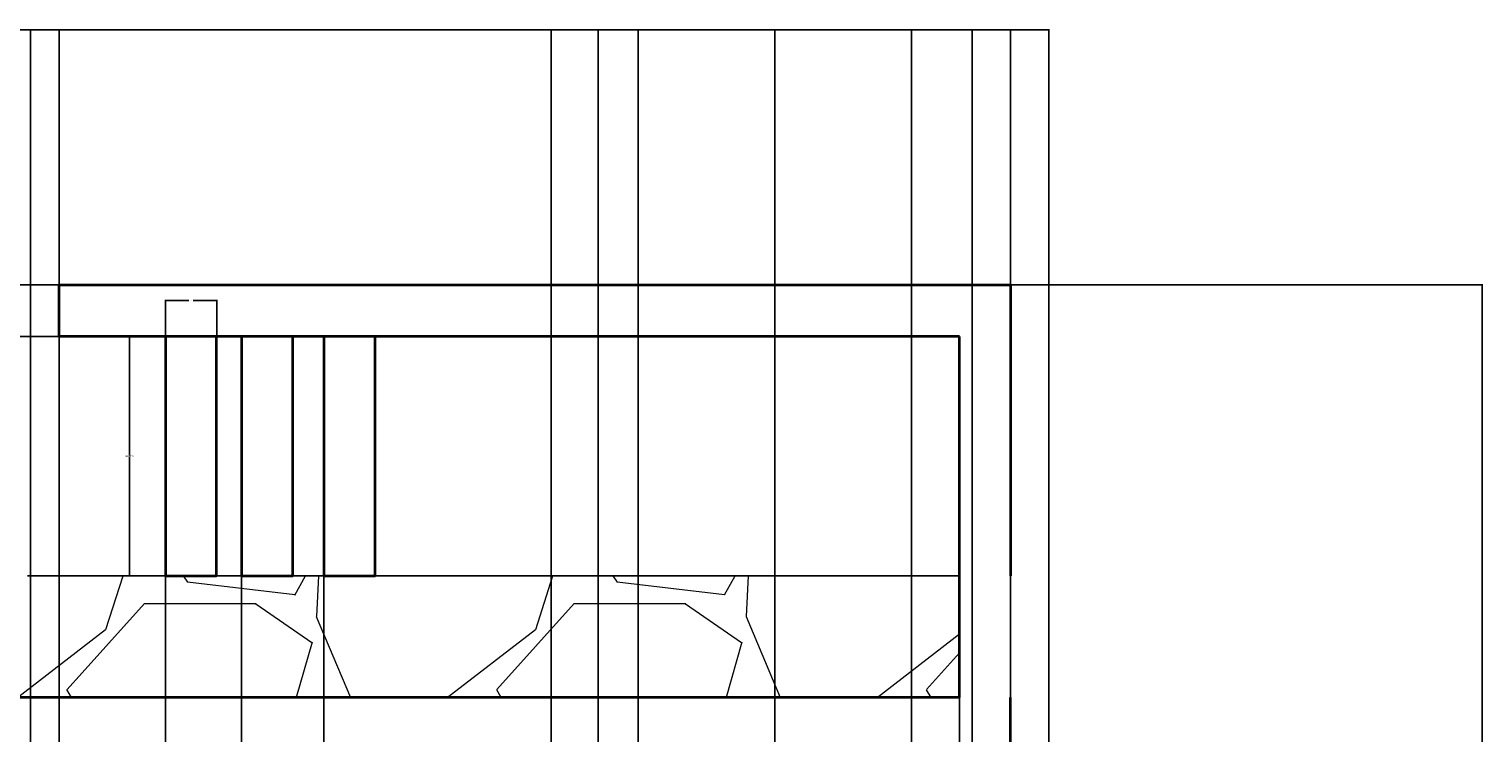
# Model space of a CAD drawing. Units: inches. Extents: x -8 to 554, y -200 to 499.
# Tile 12 of 12: x 216 to 554, y 335 to 499. Entities that reach past the tile are written whole.
import ezdxf

# ---------------------------------------------------------------- set-up
doc = ezdxf.new("R2010")
doc.units = ezdxf.units.IN
doc.header["$MEASUREMENT"] = 0
for name, color, linetype, lineweight in [('A-ANNO-DIMS', 2, 'Continuous', 18), ('A-FLOR', 7, 'Continuous', 35), ('A-ROOF', 7, 'Continuous', 35), ('A-WALL', 7, 'Continuous', 35), ('A-WALL-PATT', 252, 'Continuous', 13), ('A-WALL-PRPT', 7, 'Continuous', 25)]:
    doc.layers.add(name, color=color, linetype=linetype, lineweight=lineweight)
doc.styles.get("Standard").update_dxf_attribs({"font": 'arial.ttf'})
doc.dimstyles.get("Standard").update_dxf_attribs({"dimtxt": 0.18, "dimasz": 0.18, "dimexe": 0.18, "dimexo": 0.0625, "dimgap": 0.09, "dimtad": 0, "dimtih": 1, "dimtoh": 1, "dimdec": 4, "dimzin": 0, "dimdsep": 46, "dimtxsty": 'Standard', "dimcen": 0.09, "dimadec": 0, "dimazin": 0, "dimtfac": 1, "dimtdec": 4, "dimtofl": 0, "dimtmove": 0, "dimatfit": 3, "dimfxl": 1, "dimtolj": 1, "dimtzin": 0, "dimarcsym": 0})

# ---------------------------------------------------------------- blocks, each defined once
blk = doc.blocks.new('ROOF-UPRIGHT-ELEV')
blk.add_lwpolyline([(0, 0), (11.94, 0), (11.94, 55.69), (0, 55.69)], close=True)
blk = doc.blocks.new('*D22')
at = {"layer": 'A-ANNO-DIMS', "color": 0, "lineweight": -2, "transparency": 16777216}
for p, q in [((247.65, 427.48), (239.18, 427.48)), ((239.36, 427.3), (239.36, 399.82)), ((239.36, 371.97), (239.36, 399.45)), ((247.65, 371.79), (239.18, 371.79))]:
    blk.add_line(p, q, dxfattribs=at)
at = {"layer": 'A-ANNO-DIMS', "color": 0, "transparency": 16777216}
for points in [[(239.33, 427.3), (239.39, 427.3), (239.36, 427.48)], [(239.33, 371.97), (239.39, 371.97), (239.36, 371.79)]]:
    blk.add_solid(points, dxfattribs=at)
at = {"layer": 'Defpoints', "color": 0, "transparency": 16777216}
for p in [(239.36, 427.48), (247.72, 427.48), (247.72, 371.79)]:
    blk.add_point(p, dxfattribs=at)
at = {"layer": 'A-ANNO-DIMS', "color": 0, "transparency": 16777216, "insert": (239.36, 399.64), "char_height": 0.18, "attachment_point": 5}
blk.add_mtext('\\A1;UPRIGHT 56 TYP.', dxfattribs=at)
blk = doc.blocks.new('*D23')
at = {"layer": 'A-ANNO-DIMS', "color": 0, "lineweight": -2, "transparency": 16777216}
for p, q in [((247.72, 427.54), (247.72, 436.01)), ((247.9, 435.83), (253.17, 435.83)), ((259.48, 435.83), (254.21, 435.83)), ((259.66, 427.54), (259.66, 436.01))]:
    blk.add_line(p, q, dxfattribs=at)
at = {"layer": 'A-ANNO-DIMS', "color": 0, "transparency": 16777216}
for points in [[(247.9, 435.86), (247.9, 435.8), (247.72, 435.83)], [(259.48, 435.86), (259.48, 435.8), (259.66, 435.83)]]:
    blk.add_solid(points, dxfattribs=at)
at = {"layer": 'Defpoints', "color": 0, "transparency": 16777216}
for p in [(259.66, 435.83), (247.72, 427.48), (259.66, 427.48)]:
    blk.add_point(p, dxfattribs=at)
at = {"layer": 'A-ANNO-DIMS', "color": 0, "transparency": 16777216, "insert": (253.69, 435.83), "char_height": 0.18, "attachment_point": 5}
blk.add_mtext('\\A1;12 TYP.', dxfattribs=at)
blk = doc.blocks.new('*D30')
at = {"layer": 'A-ANNO-DIMS', "color": 0, "lineweight": -2, "transparency": 16777216}
for p, q in [((444.4, 439.48), (554.26, 439.48)), ((554.08, 439.3), (554.08, 163.66)), ((554.08, -112.34), (554.08, 163.3)), ((446.15, -112.52), (554.26, -112.52))]:
    blk.add_line(p, q, dxfattribs=at)
at = {"layer": 'A-ANNO-DIMS', "color": 0, "transparency": 16777216}
for points in [[(554.05, 439.3), (554.11, 439.3), (554.08, 439.48)], [(554.05, -112.34), (554.11, -112.34), (554.08, -112.52)]]:
    blk.add_solid(points, dxfattribs=at)
at = {"layer": 'Defpoints', "color": 0, "transparency": 16777216}
for p in [(444.34, 439.48), (446.09, -112.52), (554.08, -112.52)]:
    blk.add_point(p, dxfattribs=at)
at = {"layer": 'A-ANNO-DIMS', "color": 0, "transparency": 16777216, "insert": (554.08, 163.48), "char_height": 0.18, "attachment_point": 5}
blk.add_mtext('\\A1;552', dxfattribs=at)
blk = doc.blocks.new('*D39')
at = {"layer": 'A-ANNO-DIMS', "color": 0, "lineweight": -2, "transparency": 16777216}
for p, q in [((223.01, 439.54), (223.01, 498.99)), ((223.19, 498.81), (333.21, 498.81)), ((444.16, 498.81), (334.14, 498.81)), ((444.34, 439.54), (444.34, 498.99))]:
    blk.add_line(p, q, dxfattribs=at)
at = {"layer": 'A-ANNO-DIMS', "color": 0, "transparency": 16777216}
for points in [[(223.19, 498.84), (223.19, 498.78), (223.01, 498.81)], [(444.16, 498.84), (444.16, 498.78), (444.34, 498.81)]]:
    blk.add_solid(points, dxfattribs=at)
at = {"layer": 'Defpoints', "color": 0, "transparency": 16777216}
for p in [(444.34, 498.81), (223.01, 439.48), (444.34, 439.48)]:
    blk.add_point(p, dxfattribs=at)
at = {"layer": 'A-ANNO-DIMS', "color": 0, "transparency": 16777216, "insert": (333.68, 498.81), "char_height": 0.18, "attachment_point": 5}
blk.add_mtext('\\A1;221.33', dxfattribs=at)
blk = doc.blocks.new('*D40')
at = {"layer": 'A-ANNO-DIMS', "color": 0, "lineweight": -2, "transparency": 16777216}
for p, q in [((222.95, 439.48), (-7.69, 439.48)), ((-7.51, 439.3), (-7.51, 433.66)), ((-7.51, 427.66), (-7.51, 433.3)), ((222.95, 427.48), (-7.69, 427.48))]:
    blk.add_line(p, q, dxfattribs=at)
at = {"layer": 'A-ANNO-DIMS', "color": 0, "transparency": 16777216}
for points in [[(-7.54, 439.3), (-7.48, 439.3), (-7.51, 439.48)], [(-7.54, 427.66), (-7.48, 427.66), (-7.51, 427.48)]]:
    blk.add_solid(points, dxfattribs=at)
at = {"layer": 'Defpoints', "color": 0, "transparency": 16777216}
for p in [(223.01, 439.48), (-7.51, 427.48), (223.01, 427.48)]:
    blk.add_point(p, dxfattribs=at)
at = {"layer": 'A-ANNO-DIMS', "color": 0, "transparency": 16777216, "insert": (-7.51, 433.48), "char_height": 0.18, "attachment_point": 5}
blk.add_mtext('\\A1;12', dxfattribs=at)
blk = doc.blocks.new('*D43')
at = {"layer": 'A-ANNO-DIMS', "color": 0, "lineweight": -2, "transparency": 16777216}
for p, q in [((168.34, 319.54), (168.34, 498.99)), ((168.52, 498.81), (192.12, 498.81)), ((216.16, 498.81), (192.56, 498.81)), ((216.34, 319.54), (216.34, 498.99))]:
    blk.add_line(p, q, dxfattribs=at)
at = {"layer": 'A-ANNO-DIMS', "color": 0, "transparency": 16777216}
for points in [[(168.52, 498.84), (168.52, 498.78), (168.34, 498.81)], [(216.16, 498.84), (216.16, 498.78), (216.34, 498.81)]]:
    blk.add_solid(points, dxfattribs=at)
at = {"layer": 'Defpoints', "color": 0, "transparency": 16777216}
for p in [(216.34, 498.81), (168.34, 319.48), (216.34, 319.48)]:
    blk.add_point(p, dxfattribs=at)
at = {"layer": 'A-ANNO-DIMS', "color": 0, "transparency": 16777216, "insert": (192.34, 498.81), "char_height": 0.18, "attachment_point": 5}
blk.add_mtext('\\A1;48', dxfattribs=at)
blk = doc.blocks.new('*D45')
at = {"layer": 'A-ANNO-DIMS', "color": 0, "lineweight": -2, "transparency": 16777216}
for p, q in [((357.7, 319.85), (357.7, 498.99)), ((357.88, 498.81), (373.22, 498.81)), ((389.34, 498.81), (374, 498.81)), ((389.52, 319.54), (389.52, 498.99))]:
    blk.add_line(p, q, dxfattribs=at)
at = {"layer": 'A-ANNO-DIMS', "color": 0, "transparency": 16777216}
for points in [[(357.88, 498.84), (357.88, 498.78), (357.7, 498.81)], [(389.34, 498.84), (389.34, 498.78), (389.52, 498.81)]]:
    blk.add_solid(points, dxfattribs=at)
at = {"layer": 'Defpoints', "color": 0, "transparency": 16777216}
for p in [(389.52, 498.81), (357.7, 319.79), (389.52, 319.48)]:
    blk.add_point(p, dxfattribs=at)
at = {"layer": 'A-ANNO-DIMS', "color": 0, "transparency": 16777216, "insert": (373.61, 498.81), "char_height": 0.18, "attachment_point": 5}
blk.add_mtext('\\A1;31.82', dxfattribs=at)
blk = doc.blocks.new('*D55')
at = {"layer": 'A-ANNO-DIMS', "color": 0, "lineweight": -2, "transparency": 16777216}
for p, q in [((204.61, -30.61), (204.61, 498.99)), ((204.79, 498.81), (328.57, 498.81)), ((453.14, 498.81), (329.36, 498.81)), ((453.32, -30.61), (453.32, 498.99))]:
    blk.add_line(p, q, dxfattribs=at)
at = {"layer": 'A-ANNO-DIMS', "color": 0, "transparency": 16777216}
for points in [[(204.79, 498.84), (204.79, 498.78), (204.61, 498.81)], [(453.14, 498.84), (453.14, 498.78), (453.32, 498.81)]]:
    blk.add_solid(points, dxfattribs=at)
at = {"layer": 'Defpoints', "color": 0, "transparency": 16777216}
for p in [(453.32, 498.81), (204.61, -30.67), (453.32, -30.67)]:
    blk.add_point(p, dxfattribs=at)
at = {"layer": 'A-ANNO-DIMS', "color": 0, "transparency": 16777216, "insert": (328.96, 498.81), "char_height": 0.18, "attachment_point": 5}
blk.add_mtext('\\A1;248.7', dxfattribs=at)
blk = doc.blocks.new('*D62')
at = {"layer": 'A-ANNO-DIMS', "color": 0, "lineweight": -2, "transparency": 16777216}
for p, q in [((189.3, 7.54), (189.3, 498.99)), ((189.48, 498.81), (263.01, 498.81)), ((337.31, 498.81), (263.78, 498.81)), ((337.49, 7.54), (337.49, 498.99))]:
    blk.add_line(p, q, dxfattribs=at)
at = {"layer": 'A-ANNO-DIMS', "color": 0, "transparency": 16777216}
for points in [[(189.48, 498.84), (189.48, 498.78), (189.3, 498.81)], [(337.31, 498.84), (337.31, 498.78), (337.49, 498.81)]]:
    blk.add_solid(points, dxfattribs=at)
at = {"layer": 'Defpoints', "color": 0, "transparency": 16777216}
for p in [(337.49, 498.81), (189.3, 7.48), (337.49, 7.48)]:
    blk.add_point(p, dxfattribs=at)
at = {"layer": 'A-ANNO-DIMS', "color": 0, "transparency": 16777216, "insert": (263.4, 498.81), "char_height": 0.18, "attachment_point": 5}
blk.add_mtext('\\A1;148.2', dxfattribs=at)
blk = doc.blocks.new('*D63')
at = {"layer": 'A-ANNO-DIMS', "color": 0, "lineweight": -2, "transparency": 16777216}
for p, q in [((337.49, -52.76), (337.49, 498.99)), ((337.67, 498.81), (342.51, 498.81)), ((348.26, 498.81), (343.42, 498.81)), ((348.44, -52.76), (348.44, 498.99))]:
    blk.add_line(p, q, dxfattribs=at)
at = {"layer": 'A-ANNO-DIMS', "color": 0, "transparency": 16777216}
for points in [[(337.67, 498.84), (337.67, 498.78), (337.49, 498.81)], [(348.26, 498.84), (348.26, 498.78), (348.44, 498.81)]]:
    blk.add_solid(points, dxfattribs=at)
at = {"layer": 'Defpoints', "color": 0, "transparency": 16777216}
for p in [(348.44, 498.81), (337.49, -52.82), (348.44, -52.82)]:
    blk.add_point(p, dxfattribs=at)
at = {"layer": 'A-ANNO-DIMS', "color": 0, "transparency": 16777216, "insert": (342.97, 498.81), "char_height": 0.18, "attachment_point": 5}
blk.add_mtext('\\A1;10.946', dxfattribs=at)
blk = doc.blocks.new('*D64')
at = {"layer": 'A-ANNO-DIMS', "color": 0, "lineweight": -2, "transparency": 16777216}
for p, q in [((337.49, 7.54), (337.49, 498.99)), ((337.67, 498.81), (379.02, 498.81)), ((421.13, 498.81), (379.78, 498.81)), ((421.31, 7.54), (421.31, 498.99))]:
    blk.add_line(p, q, dxfattribs=at)
at = {"layer": 'A-ANNO-DIMS', "color": 0, "transparency": 16777216}
for points in [[(337.67, 498.84), (337.67, 498.78), (337.49, 498.81)], [(421.13, 498.84), (421.13, 498.78), (421.31, 498.81)]]:
    blk.add_solid(points, dxfattribs=at)
at = {"layer": 'Defpoints', "color": 0, "transparency": 16777216}
for p in [(421.31, 498.81), (337.49, 7.48), (421.31, 7.48)]:
    blk.add_point(p, dxfattribs=at)
at = {"layer": 'A-ANNO-DIMS', "color": 0, "transparency": 16777216, "insert": (379.4, 498.81), "char_height": 0.18, "attachment_point": 5}
blk.add_mtext('\\A1;83.81', dxfattribs=at)
blk = doc.blocks.new('*D65')
at = {"layer": 'A-ANNO-DIMS', "color": 0, "lineweight": -2, "transparency": 16777216}
for p, q in [((421.31, 7.54), (421.31, 498.99)), ((421.49, 498.81), (428, 498.81)), ((435.29, 498.81), (428.77, 498.81)), ((435.47, 7.54), (435.47, 498.99))]:
    blk.add_line(p, q, dxfattribs=at)
at = {"layer": 'A-ANNO-DIMS', "color": 0, "transparency": 16777216}
for points in [[(421.49, 498.84), (421.49, 498.78), (421.31, 498.81)], [(435.29, 498.84), (435.29, 498.78), (435.47, 498.81)]]:
    blk.add_solid(points, dxfattribs=at)
at = {"layer": 'Defpoints', "color": 0, "transparency": 16777216}
for p in [(435.47, 498.81), (421.31, 7.48), (435.47, 7.48)]:
    blk.add_point(p, dxfattribs=at)
at = {"layer": 'A-ANNO-DIMS', "color": 0, "transparency": 16777216, "insert": (428.39, 498.81), "char_height": 0.18, "attachment_point": 5}
blk.add_mtext('\\A1;14.16', dxfattribs=at)
blk = doc.blocks.new('*D67')
at = {"layer": 'A-ANNO-DIMS', "color": 0, "lineweight": -2, "transparency": 16777216}
for p, q in [((223.01, 427.42), (223.01, -199.97)), ((247.72, 427.42), (247.72, -199.97)), ((223.19, -199.79), (234.9, -199.79)), ((247.54, -199.79), (235.83, -199.79))]:
    blk.add_line(p, q, dxfattribs=at)
at = {"layer": 'A-ANNO-DIMS', "color": 0, "transparency": 16777216}
for points in [[(223.19, -199.76), (223.19, -199.82), (223.01, -199.79)], [(247.54, -199.76), (247.54, -199.82), (247.72, -199.79)]]:
    blk.add_solid(points, dxfattribs=at)
at = {"layer": 'Defpoints', "color": 0, "transparency": 16777216}
for p in [(223.01, 427.48), (247.72, 427.48), (247.72, -199.79)]:
    blk.add_point(p, dxfattribs=at)
at = {"layer": 'A-ANNO-DIMS', "color": 0, "transparency": 16777216, "insert": (235.36, -199.79), "char_height": 0.18, "attachment_point": 5}
blk.add_mtext('\\A1;24.705', dxfattribs=at)
blk = doc.blocks.new('*D68')
at = {"layer": 'A-ANNO-DIMS', "color": 0, "lineweight": -2, "transparency": 16777216}
for p, q in [((247.72, 371.73), (247.72, -199.97)), ((265.46, 371.73), (265.46, -199.97)), ((247.9, -199.79), (256.13, -199.79)), ((265.28, -199.79), (257.04, -199.79))]:
    blk.add_line(p, q, dxfattribs=at)
at = {"layer": 'A-ANNO-DIMS', "color": 0, "transparency": 16777216}
for points in [[(247.9, -199.76), (247.9, -199.82), (247.72, -199.79)], [(265.28, -199.76), (265.28, -199.82), (265.46, -199.79)]]:
    blk.add_solid(points, dxfattribs=at)
at = {"layer": 'Defpoints', "color": 0, "transparency": 16777216}
for p in [(247.72, 371.79), (265.46, 371.79), (265.46, -199.79)]:
    blk.add_point(p, dxfattribs=at)
at = {"layer": 'A-ANNO-DIMS', "color": 0, "transparency": 16777216, "insert": (256.59, -199.79), "char_height": 0.18, "attachment_point": 5}
blk.add_mtext('\\A1;17.744', dxfattribs=at)
blk = doc.blocks.new('*D69')
at = {"layer": 'A-ANNO-DIMS', "color": 0, "lineweight": -2, "transparency": 16777216}
for p, q in [((265.46, 371.73), (265.46, -199.97)), ((284.57, 371.73), (284.57, -199.97)), ((265.64, -199.79), (274.65, -199.79)), ((284.39, -199.79), (275.38, -199.79))]:
    blk.add_line(p, q, dxfattribs=at)
at = {"layer": 'A-ANNO-DIMS', "color": 0, "transparency": 16777216}
for points in [[(265.64, -199.76), (265.64, -199.82), (265.46, -199.79)], [(284.39, -199.76), (284.39, -199.82), (284.57, -199.79)]]:
    blk.add_solid(points, dxfattribs=at)
at = {"layer": 'Defpoints', "color": 0, "transparency": 16777216}
for p in [(265.46, 371.79), (284.57, 371.79), (284.57, -199.79)]:
    blk.add_point(p, dxfattribs=at)
at = {"layer": 'A-ANNO-DIMS', "color": 0, "transparency": 16777216, "insert": (275.01, -199.79), "char_height": 0.18, "attachment_point": 5}
blk.add_mtext('\\A1;19.11', dxfattribs=at)
blk = doc.blocks.new('*D71')
at = {"layer": 'A-ANNO-DIMS', "color": 0, "lineweight": -2, "transparency": 16777216}
for p, q in [((444.34, 439.42), (444.34, -199.97)), ((432.52, 427.42), (432.52, -199.97)), ((432.7, -199.79), (437.97, -199.79)), ((444.16, -199.79), (438.89, -199.79))]:
    blk.add_line(p, q, dxfattribs=at)
at = {"layer": 'A-ANNO-DIMS', "color": 0, "transparency": 16777216}
for points in [[(432.7, -199.76), (432.7, -199.82), (432.52, -199.79)], [(444.16, -199.76), (444.16, -199.82), (444.34, -199.79)]]:
    blk.add_solid(points, dxfattribs=at)
at = {"layer": 'Defpoints', "color": 0, "transparency": 16777216}
for p in [(444.34, 439.48), (432.52, 427.48), (444.34, -199.79)]:
    blk.add_point(p, dxfattribs=at)
at = {"layer": 'A-ANNO-DIMS', "color": 0, "transparency": 16777216, "insert": (438.43, -199.79), "char_height": 0.18, "attachment_point": 5}
blk.add_mtext('\\A1;11.825', dxfattribs=at)

msp = doc.modelspace()

# ---------------------------------------------------------------- hatches: boundary and pattern name
at = {"layer": 'A-WALL-PATT'}
h = msp.add_hatch(dxfattribs=at)
h.set_pattern_fill('GRAVEL', color=256, scale=100)
h.set_pattern_definition([(228.0128, (-45.809, 19.688), (-800, -900), [13.4536, -1331.909]), (184.9697, (-54.8087, 9.688), (1200, 100), [23.0868, -2285.5925]), (132.5104, (-77.809, 7.688), (1000, -1100), [16.279, -1611.6033]), (267.2737, (-116.8087, -17.312), (100, 2000), [21.0238, -2081.3558]), (292.83365, (-117.8087, -38.312), (-500, 1200), [20.6155, -2040.9373]), (357.2737, (-109.8087, -57.312), (-2000, 100), [21.0238, -2081.3558]), (37.69424, (-88.8087, -58.3118), (-1300, -1000), [27.803, -2752.4849]), (72.2553, (-66.8087, -41.312), (700, 2200), [26.2488, -2598.632]), (121.4296, (-58.8087, -16.312), (-800, 1300), [21.095, -2088.4073]), (175.2364, (-69.809, 1.688), (1100, -100), [24.083, -1180.076]), (222.39744, (-93.8087, 3.6882), (-1200, -1100), [31.1448, -3083.3375]), (138.814, (-17.809, -18.312), (-700, 600), [10.63, -1052.3845]), (171.4692, (-25.8087, -11.312), (1300, -200), [20.2237, -2002.151]), (225, (-45.81, -8.31), (-1e-14, -100), [14.142, -127.279]), (203.1986, (-52.809, 3.688), (500, 200), [7.616, -753.9615]), (291.8014, (-59.809, 0.688), (-100, 300), [10.77, -527.746]), (30.9638, (-55.809, -9.312), (300, 200), [17.493, -565.602]), (161.565, (-40.81, -0.312), (200, -100), [12.649, -303.579]), (16.3895, (-117.8087, 0.688), (1000, 300), [17.72, -1754.2845]), (70.3462, (-100.809, 5.688), (-400, -1100), [14.866, -1471.741]), (293.1986, (-40.809, 19.688), (-200, 500), [15.2315, -746.346]), (343.6105, (-34.8087, 5.688), (-1000, 300), [17.72, -1754.2845]), (339.444, (-117.809, -61.312), (-500, 200), [17.088, -837.3124]), (294.7751, (-101.809, -67.312), (-500, 1100), [14.318, -1417.4643]), (66.8014, (-39.809, -80.312), (200, 500), [15.2315, -746.346]), (17.354, (-33.809, -66.312), (-1300, -400), [16.763, -1659.5424]), (69.444, (-88.809, -80.312), (-200, -500), [8.544, -845.8564]), (101.31, (-45.809, -80.312), (-100, 400), [5.099, -504.803]), (165.9638, (-46.809, -75.312), (300, -100), [20.6155, -391.695]), (186.009, (-66.8087, -70.312), (1000, 100), [19.105, -1891.3923]), (303.69, (-55.81, -18.312), (-100, 200), [14.422, -346.133]), (353.1572, (-47.8087, -30.312), (1700, -200), [25.1794, -2492.7563]), (60.9454, (-22.809, -33.312), (-400, -700), [10.2956, -1019.2674]), (90, (-17.81, -24.31), (-100, 100), [6, -94]), (120.2564, (-68.809, -67.312), (400, -700), [13.8924, -1375.352]), (48.0128, (-75.809, -55.312), (800, 900), [26.907, -1318.455]), (0, (-57.81, -35.31), (100, 100), [26, -74]), (325.3048, (-31.809, -35.312), (1000, -700), [15.8114, -1565.3274]), (254.0546, (-18.809, -44.312), (-100, -400), [14.56, -713.451]), (207.646, (-22.8087, -58.312), (-1900, -1000), [23.7065, -2346.9474]), (175.4261, (-43.8087, -69.312), (-1300, 100), [25.08, -2482.9073])])
h.paths.add_polyline_path([(48.6882, -52.5186), (24.3421, -52.5186), (24.3421, -112.5186), (48.6882, -112.5186)])
h.paths.add_polyline_path([(212.2282, -52.5186), (140.2282, -52.5186), (128.2282, -52.5186), (128.2282, -112.5186), (140.2282, -112.5186), (140.2282, -64.9665), (202.9211, -64.9665), (202.9211, -112.5186), (212.2282, -112.5186)])
h.paths.add_polyline_path([(312.3421, 49.7921), (216.3421, 49.7921), (216.3421, 19.4814), (312.3421, 19.4814)])
h.paths.add_polyline_path([(312.3421, 157.7921), (216.3421, 157.7921), (216.3421, 127.4814), (312.3421, 127.4814)])
h.paths.add_polyline_path([(312.3421, 265.7921), (216.3421, 265.7921), (216.3421, 235.4814), (312.3421, 235.4814)])
h.paths.add_polyline_path([(432.5174, 371.7921), (215.6778, 371.7921), (215.6778, 368.5162), (215.6778, 357.6367), (35.7874, 357.6367), (35.7874, 360.9127), (35.7874, 371.7921), (24.3421, 371.7921), (24.3421, 343.4814), (35.7874, 343.4814), (432.5174, 343.4814)])

# ---------------------------------------------------------------- linework, layer by layer
at = {"layer": 'A-FLOR'}
msp.add_line((432.5174, 343.4814), (24.3421, 343.4814), dxfattribs=at)
at = {"layer": 'A-ROOF'}
for p, q in [((223.0104, 427.4814), (223.0104, 439.4814)), ((223.0104, 439.4814), (444.3421, 439.4814)), ((444.3421, 439.4814), (444.3421, 371.7921)), ((432.5174, 427.4814), (223.0104, 427.4814)), ((432.5174, 343.4814), (432.5174, 427.4814))]:
    msp.add_line(p, q, dxfattribs=at)
at = {"layer": 'A-WALL'}
msp.add_line((444.3421, 223.4814), (444.3421, 343.4814), dxfattribs=at)
at = {"layer": 'A-WALL-PRPT'}
for p, q in [((432.5174, 371.7921), (215.6778, 371.7921)), ((444.3421, 371.7921), (444.3421, 343.4814))]:
    msp.add_line(p, q, dxfattribs=at)
msp.add_lwpolyline([(432.5174, 343.4814), (432.5174, 371.7921)], dxfattribs=at)

# ---------------------------------------------------------------- block references
at = {"layer": 'A-ROOF'}
for p in [(247.7159, 371.7921), (265.4598, 371.7921), (284.5686, 371.7921)]:
    msp.add_blockref('ROOF-UPRIGHT-ELEV', p, dxfattribs=at)

# ---------------------------------------------------------------- dimensions: what is measured, and where the dimension line sits
at = {"layer": 'A-ANNO-DIMS'}
for base, p1, p2, override, picture, middle in [((216.3421, 498.8091), (168.3421, 319.4814), (216.3421, 319.4814), {"dimdec": 0, "dimlfac": 1, "dimrnd": 0, "dimzin": 0, "dimdsep": 46, "dimlunit": 2}, '*D43', (192.3421, 498.8091)), ((337.4923, 498.8091), (189.3049, 7.4814), (337.4923, 7.4814), {"dimdec": 1, "dimlfac": 1, "dimrnd": 0, "dimzin": 0, "dimdsep": 46, "dimlunit": 2}, '*D62', (263.3986, 498.8091)), ((453.3222, 498.8091), (204.6055, -30.6677), (453.3222, -30.6677), {"dimdec": 1, "dimlfac": 1, "dimrnd": 0, "dimzin": 0, "dimdsep": 46, "dimlunit": 2}, '*D55', (328.9639, 498.8091)), ((444.3421, 498.8091), (223.0104, 439.4814), (444.3421, 439.4814), {"dimdec": 2, "dimlfac": 1, "dimrnd": 0, "dimzin": 0, "dimdsep": 46, "dimlunit": 2}, '*D39', (333.6762, 498.8091)), ((348.4381, 498.8091), (337.4923, -52.8231), (348.4381, -52.8231), {"dimdec": 3, "dimlfac": 1, "dimrnd": 0, "dimzin": 0, "dimdsep": 46, "dimlunit": 2}, '*D63', (342.9652, 498.8091)), ((421.3053, 498.8091), (337.4923, 7.4814), (421.3053, 7.4814), {"dimdec": 2, "dimlfac": 1, "dimrnd": 0, "dimzin": 0, "dimdsep": 46, "dimlunit": 2}, '*D64', (379.3988, 498.8091)), ((389.5174, 498.8091), (357.699, 319.788), (389.5174, 319.4814), {"dimdec": 2, "dimlfac": 1, "dimrnd": 0, "dimzin": 0, "dimdsep": 46, "dimlunit": 2}, '*D45', (373.6082, 498.8091)), ((435.4655, 498.8091), (421.3053, 7.4814), (435.4655, 7.4814), {"dimdec": 2, "dimlfac": 1, "dimrnd": 0, "dimzin": 0, "dimdsep": 46, "dimlunit": 2}, '*D65', (428.3854, 498.8091)), ((444.3421, -199.7912), (432.5174, 427.4814), (444.3421, 439.4814), {"dimdec": 3, "dimlfac": 1, "dimrnd": 0, "dimzin": 0, "dimdsep": 46, "dimlunit": 2}, '*D71', (438.4297, -199.7912)), ((247.71587, -199.79119), (223.01039, 427.48136), (247.71587, 427.48136), {"dimdec": 3, "dimlfac": 1, "dimrnd": 0, "dimzin": 0, "dimdsep": 46, "dimlunit": 2}, '*D67', (235.36313, -199.79119)), ((265.4598, -199.7912), (247.7159, 371.7921), (265.4598, 371.7921), {"dimdec": 3, "dimlfac": 1, "dimrnd": 0, "dimzin": 0, "dimdsep": 46, "dimlunit": 2}, '*D68', (256.5878, -199.7912)), ((284.5686, -199.7912), (265.4598, 371.7921), (284.5686, 371.7921), {"dimdec": 2, "dimlfac": 1, "dimrnd": 0, "dimzin": 0, "dimdsep": 46, "dimlunit": 2}, '*D69', (275.0142, -199.7912))]:
    dim = msp.add_linear_dim(base=base, p1=p1, p2=p2, dimstyle='Standard', override=override, dxfattribs=at)
    dim.commit()
    dim.dimension.update_dxf_attribs({"geometry": picture, "text_midpoint": middle})
for base, p1, p2, picture, middle in [((-7.5079, 427.4814), (223.0104, 439.4814), (223.0104, 427.4814), '*D40', (-7.5079, 433.4814)), ((554.0833, -112.5186), (444.3421, 439.4814), (446.0855, -112.5186), '*D30', (554.0833, 163.4814))]:
    dim = msp.add_linear_dim(base=base, p1=p1, p2=p2, angle=90, dimstyle='Standard', override={"dimdec": 0, "dimlfac": 1, "dimrnd": 0, "dimzin": 0, "dimdsep": 46, "dimlunit": 2}, dxfattribs=at)
    dim.commit()
    dim.dimension.update_dxf_attribs({"geometry": picture, "text_midpoint": middle})
dim = msp.add_linear_dim(base=(259.6589, 435.8347), p1=(247.7159, 427.4814), p2=(259.6589, 427.4814), text='<> TYP.', dimstyle='Standard', override={"dimdec": 0, "dimlfac": 1, "dimrnd": 0, "dimzin": 0, "dimdsep": 46, "dimlunit": 2}, dxfattribs=at)
dim.commit()
dim.dimension.update_dxf_attribs({"geometry": '*D23', "text_midpoint": (253.6874, 435.8347)})
dim = msp.add_linear_dim(base=(239.3625, 427.4814), p1=(247.7159, 371.7921), p2=(247.7159, 427.4814), angle=90, text='UPRIGHT <> TYP.', dimstyle='Standard', override={"dimdec": 0, "dimlfac": 1, "dimrnd": 0, "dimzin": 0, "dimdsep": 46, "dimlunit": 2}, dxfattribs=at)
dim.commit()
dim.dimension.update_dxf_attribs({"geometry": '*D22', "text_midpoint": (239.3625, 399.6367)})

doc.saveas('drawing.dxf')
